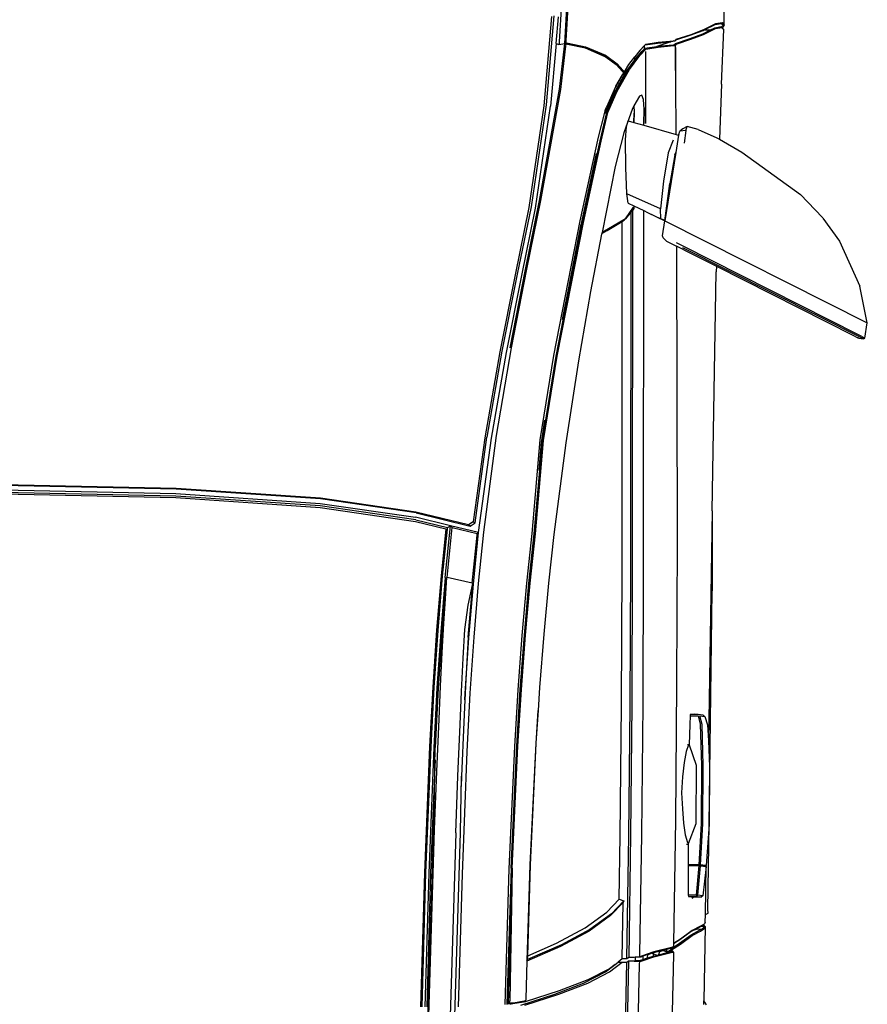
# Model space of a CAD drawing. Units: inches. Extents: x 0 to 4258, y 0 to 3769.
# Tile 11 of 30: x 3761 to 3796, y 3042 to 3082. Entities that reach past the tile are written whole.
import ezdxf

# ---------------------------------------------------------------- set-up
doc = ezdxf.new("R2010")
doc.units = ezdxf.units.IN
doc.header["$MEASUREMENT"] = 0
doc.layers.get('0').update_dxf_attribs({"color": 16})
doc.layers.add('C-PKNG-VEHI', color=8, linetype='Continuous', lineweight=18)
doc.layers.add('Edges', color=250, linetype='Continuous')

# ---------------------------------------------------------------- blocks, each defined once
blk = doc.blocks.new('Nissan Qashqai pl')
at = {"layer": 'Edges'}
for p, q in [((8.8918, 12.7444), (9.0186, 12.9956)), ((9.0386, 12.9907), (8.9254, 12.7664)), ((9.0186, 12.9956), (8.9731, 12.9865)), ((9.0374, 12.9925), (9.0186, 12.9956)), ((9.0356, 12.9888), (9.0333, 12.9845)), ((9.0356, 12.9888), (9.0374, 12.9925)), ((9.0386, 12.9907), (9.0374, 12.9925)), ((9.0376, 12.985), (9.0386, 12.9907)), ((8.9173, 12.961), (8.9731, 12.9865)), ((9.0333, 12.9845), (8.9232, 12.7662)), ((8.9483, 12.8082), (9.0343, 12.9785)), ((9.0343, 12.9785), (9.0347, 12.9794)), ((9.0347, 12.9794), (9.0362, 12.9822)), ((9.0362, 12.9822), (9.037, 12.9838)), ((9.0371, 12.9841), (9.037, 12.9838)), ((9.0371, 12.9841), (9.0376, 12.985)), ((9.0376, 12.985), (9.0371, 12.9847)), ((8.8885, 12.9405), (8.9173, 12.961)), ((8.8591, 12.9127), (8.8879, 12.94)), ((8.8885, 12.9405), (8.8879, 12.94)), ((8.8066, 12.84), (8.8591, 12.9127)), ((8.7908, 12.812), (8.8066, 12.84)), ((8.6489, 12.8179), (8.5719, 12.8193)), ((8.646, 12.8153), (8.6489, 12.8179)), ((8.6489, 12.8179), (8.6527, 12.8156)), ((8.6547, 12.8176), (8.6537, 12.8167)), ((8.7222, 12.8144), (8.6547, 12.8176)), ((8.646, 12.8153), (8.646, 12.8153)), ((8.6472, 12.8076), (8.646, 12.8153)), ((8.647, 12.8142), (8.6498, 12.8168)), ((8.6482, 12.8067), (8.647, 12.8142)), ((8.6546, 12.7926), (8.6472, 12.8076)), ((8.655, 12.7929), (8.6482, 12.8067)), ((8.6498, 12.8168), (8.6524, 12.8153)), ((8.651, 12.814), (8.652, 12.815)), ((8.6524, 12.8064), (8.651, 12.814)), ((8.652, 12.815), (8.6524, 12.8153)), ((8.6534, 12.8073), (8.652, 12.815)), ((8.6524, 12.8153), (8.6527, 12.8156)), ((8.655, 12.801), (8.6524, 12.8064)), ((8.6527, 12.8156), (8.6537, 12.8167)), ((8.6608, 12.7921), (8.6534, 12.8073)), ((8.6537, 12.8167), (8.6537, 12.8166)), ((8.7222, 12.8144), (8.7908, 12.812)), ((8.7785, 12.7855), (8.7891, 12.8089)), ((8.7891, 12.8089), (8.7908, 12.812)), ((8.928, 12.7679), (8.9483, 12.8082)), ((8.9483, 12.8082), (8.9552, 12.8081)), ((9.2517, 12.8031), (8.9552, 12.8081)), ((8.6606, 12.7768), (8.6546, 12.7926)), ((8.6598, 12.7913), (8.655, 12.801)), ((8.655, 12.7929), (8.655, 12.801)), ((8.6556, 12.7918), (8.655, 12.7929)), ((8.655, 12.7922), (8.655, 12.7929)), ((9.2517, 12.8031), (9.351, 12.803)), ((9.2517, 12.8031), (9.5372, 12.7983)), ((9.641, 12.7991), (9.351, 12.803)), ((9.5052, 12.7918), (9.5069, 12.7941)), ((9.5061, 12.7878), (9.5069, 12.7941)), ((9.5069, 12.7941), (9.5176, 12.7972)), ((9.5176, 12.7972), (9.5372, 12.7983)), ((9.5372, 12.7983), (9.5689, 12.7999)), ((9.5689, 12.7999), (9.641, 12.7991)), ((9.641, 12.7991), (9.6921, 12.7956)), ((9.7466, 12.7978), (9.641, 12.7991)), ((9.692, 12.7943), (9.6913, 12.7886)), ((9.6921, 12.7956), (9.692, 12.7943)), ((9.6922, 12.7943), (9.692, 12.7943)), ((9.6922, 12.7943), (9.6921, 12.7956)), ((9.7526, 12.7946), (9.6921, 12.7956)), ((9.6922, 12.7885), (9.693, 12.7955)), ((9.6922, 12.7885), (9.6922, 12.7943)), ((9.693, 12.7955), (9.7296, 12.7914)), ((9.7511, 12.7979), (9.7466, 12.7978)), ((9.7526, 12.7946), (9.7511, 12.7979)), ((9.7623, 12.7945), (9.7526, 12.7946)), ((9.7623, 12.7945), (9.7643, 12.7937)), ((9.7643, 12.7937), (9.7652, 12.7927)), ((9.7643, 12.7937), (9.7648, 12.7929)), ((9.7648, 12.7929), (9.7648, 12.7929)), ((9.7648, 12.7929), (9.7664, 12.7902)), ((9.7652, 12.7927), (9.7665, 12.7907)), ((9.7667, 12.7933), (9.7665, 12.7907)), ((9.7677, 12.7944), (9.7667, 12.7933)), ((9.7676, 12.7931), (9.7667, 12.7933)), ((9.7673, 12.7899), (9.7676, 12.7931)), ((9.769, 12.7926), (9.7676, 12.7931)), ((9.7677, 12.7944), (9.7677, 12.7944)), ((9.77, 12.7936), (9.7677, 12.7944)), ((9.7677, 12.7944), (9.8598, 12.7928)), ((9.7712, 12.7892), (9.769, 12.7926)), ((9.7734, 12.7884), (9.77, 12.7936)), ((9.8598, 12.7928), (9.8614, 12.7937)), ((9.8643, 12.7927), (9.8598, 12.7928)), ((9.8614, 12.7937), (9.8647, 12.7956)), ((8.6616, 12.7758), (8.6556, 12.7918)), ((8.6657, 12.7758), (8.6598, 12.7913)), ((8.6667, 12.7767), (8.6608, 12.7921)), ((8.7785, 12.7855), (8.7751, 12.7719)), ((9.5037, 12.7806), (9.5045, 12.7814)), ((9.5052, 12.7918), (9.5044, 12.7856)), ((9.5044, 12.7856), (9.5045, 12.7814)), ((9.5045, 12.7814), (9.5045, 12.7759)), ((9.5168, 12.7904), (9.5061, 12.7878)), ((9.5061, 12.7856), (9.5167, 12.7883)), ((9.5063, 12.7755), (9.5061, 12.7856)), ((9.5167, 12.7883), (9.5679, 12.7899)), ((9.5679, 12.792), (9.5168, 12.7904)), ((9.5678, 12.7837), (9.5426, 12.7747)), ((9.64, 12.7831), (9.5678, 12.7837)), ((9.6401, 12.7914), (9.5679, 12.792)), ((9.5679, 12.7899), (9.64, 12.7892)), ((9.64, 12.7892), (9.6912, 12.7865)), ((9.6645, 12.7737), (9.64, 12.7831)), ((9.6913, 12.7886), (9.6401, 12.7914)), ((9.6912, 12.7811), (9.6911, 12.7796)), ((9.6913, 12.7886), (9.6912, 12.7865)), ((9.6912, 12.7865), (9.6912, 12.7811)), ((9.692, 12.7811), (9.6912, 12.7811)), ((9.692, 12.7811), (9.6921, 12.7864)), ((9.692, 12.7796), (9.692, 12.7811)), ((9.6922, 12.7885), (9.6921, 12.7864)), ((9.6921, 12.7864), (9.7288, 12.7832)), ((9.7288, 12.7854), (9.6922, 12.7885)), ((9.7288, 12.7832), (9.7287, 12.7734)), ((9.7296, 12.7914), (9.7288, 12.7854)), ((9.7306, 12.7834), (9.7288, 12.7854)), ((9.7288, 12.7854), (9.7288, 12.7832)), ((9.7288, 12.7832), (9.7306, 12.7834)), ((9.7296, 12.7914), (9.7314, 12.7895)), ((9.7305, 12.7738), (9.7306, 12.7834)), ((9.7306, 12.7834), (9.7314, 12.7895)), ((9.7314, 12.7895), (9.7313, 12.7798)), ((9.7665, 12.7904), (9.7664, 12.7902)), ((9.7664, 12.7902), (9.7674, 12.7885)), ((9.7665, 12.7907), (9.7676, 12.7889)), ((9.7673, 12.7897), (9.7673, 12.7899)), ((9.7673, 12.7897), (9.7676, 12.7889)), ((9.7674, 12.7885), (9.7728, 12.7781)), ((9.7676, 12.7889), (9.7684, 12.7875)), ((9.7676, 12.7887), (9.7678, 12.7882)), ((9.7684, 12.7875), (9.7717, 12.781)), ((9.7707, 12.7848), (9.7709, 12.7893)), ((9.7717, 12.781), (9.7707, 12.7848)), ((9.7709, 12.7893), (9.7712, 12.7892)), ((9.7724, 12.7874), (9.7712, 12.7892)), ((9.7717, 12.781), (9.7738, 12.7771)), ((9.7778, 12.777), (9.7724, 12.7874)), ((9.7788, 12.778), (9.7734, 12.7884)), ((8.6667, 12.7584), (8.6606, 12.7768)), ((8.6675, 12.758), (8.6616, 12.7758)), ((8.6718, 12.7574), (8.6657, 12.7758)), ((8.6728, 12.7584), (8.6667, 12.7767)), ((8.7751, 12.7719), (8.7779, 12.7668)), ((8.7798, 12.7703), (8.7751, 12.7719)), ((8.7798, 12.7703), (8.7807, 12.763)), ((8.7798, 12.7703), (8.7954, 12.7683)), ((9.5045, 12.7759), (9.5063, 12.7755)), ((9.5063, 12.7755), (9.5168, 12.7751)), ((9.5168, 12.7751), (9.5423, 12.7746)), ((9.5423, 12.7746), (9.5422, 12.7736)), ((9.5422, 12.7736), (9.5422, 12.7725)), ((9.5422, 12.7736), (9.5424, 12.7735)), ((9.5426, 12.7747), (9.5423, 12.7746)), ((9.5426, 12.7747), (9.5424, 12.7735)), ((9.5424, 12.7735), (9.5503, 12.7706)), ((9.5503, 12.7706), (9.5641, 12.7681)), ((9.6395, 12.7676), (9.654, 12.7697)), ((9.654, 12.7697), (9.6633, 12.7726)), ((9.6633, 12.7726), (9.6645, 12.7737)), ((9.6655, 12.7733), (9.6645, 12.7737)), ((9.6655, 12.7733), (9.6911, 12.7732)), ((9.6655, 12.7713), (9.6655, 12.7733)), ((9.6911, 12.7796), (9.6911, 12.7732)), ((9.6911, 12.7732), (9.692, 12.7733)), ((9.692, 12.7733), (9.692, 12.7796)), ((9.692, 12.7733), (9.7287, 12.7734)), ((9.7287, 12.7734), (9.7305, 12.7738)), ((9.7305, 12.7738), (9.7313, 12.7798)), ((9.733, 12.7782), (9.7313, 12.7798)), ((9.7728, 12.7781), (9.7832, 12.7637)), ((9.7738, 12.7771), (9.7842, 12.7627)), ((9.7883, 12.7626), (9.7778, 12.777)), ((9.7894, 12.7636), (9.7788, 12.778)), ((8.6675, 12.758), (8.6667, 12.7584)), ((8.6679, 12.7578), (8.6675, 12.758)), ((8.6676, 12.7576), (8.6675, 12.7576)), ((8.6675, 12.7576), (8.6675, 12.7576)), ((8.6675, 12.7576), (8.6676, 12.7576)), ((8.6676, 12.7576), (8.6677, 12.7576)), ((8.6677, 12.7576), (8.6677, 12.7576)), ((8.6677, 12.7576), (8.6682, 12.7576)), ((8.6682, 12.7576), (8.6679, 12.7578)), ((8.6682, 12.7576), (8.6692, 12.7566)), ((8.6682, 12.7572), (8.6682, 12.7576)), ((8.6684, 12.7554), (8.6682, 12.7572)), ((8.6682, 12.7572), (8.6692, 12.7566)), ((8.6692, 12.7566), (8.6697, 12.7519)), ((8.6729, 12.7568), (8.6718, 12.7574)), ((8.674, 12.7578), (8.6728, 12.7584)), ((8.6733, 12.7566), (8.6729, 12.7568)), ((8.6735, 12.7544), (8.6733, 12.7566)), ((8.6742, 12.7576), (8.674, 12.7578)), ((8.6742, 12.7584), (8.6743, 12.7582)), ((8.6744, 12.755), (8.6742, 12.7576)), ((8.6744, 12.7576), (8.6742, 12.7576)), ((8.6744, 12.7578), (8.6744, 12.7576)), ((8.6773, 12.7577), (8.6744, 12.7576)), ((8.6791, 12.7578), (8.677, 12.7578)), ((8.6791, 12.7577), (8.6773, 12.7577)), ((8.7205, 12.7579), (8.6791, 12.7578)), ((8.6791, 12.7577), (8.6791, 12.7578)), ((8.6878, 12.7577), (8.6791, 12.7578)), ((8.6878, 12.7577), (8.6791, 12.7577)), ((8.6878, 12.7577), (8.6878, 12.7577)), ((8.6911, 12.7577), (8.6878, 12.7577)), ((8.7205, 12.7579), (8.6911, 12.7577)), ((8.7849, 12.7582), (8.7205, 12.7579)), ((8.7734, 12.7181), (8.7849, 12.7582)), ((8.7779, 12.7668), (8.7807, 12.763)), ((8.7849, 12.7615), (8.7807, 12.763)), ((8.7849, 12.7615), (8.7858, 12.7613)), ((8.7849, 12.7582), (8.7856, 12.7608)), ((8.7858, 12.7613), (8.7856, 12.7608)), ((8.7858, 12.7613), (8.807, 12.758)), ((8.8102, 12.7568), (8.807, 12.758)), ((8.807, 12.758), (8.8918, 12.7444)), ((8.8102, 12.7568), (8.8455, 12.7506)), ((8.9171, 12.7464), (8.9233, 12.7586)), ((8.9232, 12.7662), (8.9194, 12.7588)), ((8.925, 12.762), (8.9233, 12.7586)), ((8.9233, 12.7586), (9.2886, 12.7594)), ((8.928, 12.7679), (8.925, 12.762)), ((9.2886, 12.7594), (9.4673, 12.7589)), ((9.4673, 12.7589), (9.6358, 12.7575)), ((9.5641, 12.7681), (9.5818, 12.766)), ((9.5818, 12.766), (9.6016, 12.7651)), ((9.6016, 12.7651), (9.6215, 12.766)), ((9.6215, 12.766), (9.6395, 12.7676)), ((9.6358, 12.7575), (9.7887, 12.7552)), ((9.7832, 12.7637), (9.7887, 12.7552)), ((9.7842, 12.7627), (9.7891, 12.7552)), ((9.7933, 12.7549), (9.7883, 12.7626)), ((9.7965, 12.7526), (9.7894, 12.7636)), ((8.6684, 12.7554), (8.6685, 12.7549)), ((8.6684, 12.755), (8.6684, 12.7554)), ((8.6703, 12.7361), (8.6684, 12.755)), ((8.6697, 12.7519), (8.6698, 12.7516)), ((8.6714, 12.7353), (8.6697, 12.7519)), ((8.6698, 12.7516), (8.6755, 12.7343)), ((8.6754, 12.7353), (8.6735, 12.7544)), ((8.6764, 12.736), (8.6744, 12.755)), ((8.7917, 12.7547), (8.8075, 12.7486)), ((8.8075, 12.7486), (8.8429, 12.7426)), ((8.8918, 12.7444), (8.8455, 12.7506)), ((8.8815, 12.7228), (8.892, 12.7444)), ((8.892, 12.7444), (8.8908, 12.7421)), ((8.8911, 12.7428), (8.8919, 12.7444)), ((8.8911, 12.7428), (8.8919, 12.7444)), ((8.8919, 12.7444), (8.8911, 12.7428)), ((8.8919, 12.7444), (8.8918, 12.7444)), ((8.892, 12.7444), (8.8919, 12.7444)), ((8.8919, 12.7444), (8.8919, 12.7444)), ((8.8919, 12.7444), (8.8919, 12.7444)), ((8.9106, 12.7413), (8.892, 12.7444)), ((8.892, 12.7444), (8.892, 12.7444)), ((8.9171, 12.7464), (8.9131, 12.7421)), ((8.9171, 12.7464), (8.917, 12.7468)), ((9.7887, 12.7552), (9.7891, 12.7552)), ((9.7891, 12.7552), (9.79, 12.7552)), ((9.79, 12.7552), (9.7931, 12.7552)), ((9.7931, 12.7552), (9.7934, 12.7535)), ((9.7931, 12.7552), (9.7933, 12.7549)), ((9.7933, 12.7549), (9.7941, 12.7541)), ((9.7934, 12.7535), (9.7938, 12.7538)), ((9.7934, 12.7535), (9.7937, 12.7524)), ((9.7937, 12.7524), (9.7992, 12.7308)), ((9.7941, 12.7541), (9.7943, 12.7535)), ((9.7955, 12.7516), (9.7943, 12.7535)), ((9.7943, 12.7535), (9.7964, 12.7453)), ((9.7963, 12.7523), (9.7955, 12.7516)), ((9.7963, 12.7523), (9.7963, 12.7524)), ((9.7964, 12.7524), (9.7963, 12.7523)), ((9.7992, 12.7476), (9.7963, 12.7523)), ((9.7967, 12.7526), (9.7964, 12.7524)), ((9.7964, 12.7525), (9.7964, 12.7524)), ((9.7964, 12.7524), (9.7996, 12.7475)), ((9.7964, 12.7453), (9.7992, 12.7476)), ((9.7964, 12.7453), (9.7973, 12.7418)), ((9.7983, 12.7541), (9.7965, 12.7526)), ((9.7965, 12.7526), (9.7967, 12.7526)), ((9.7977, 12.7535), (9.7967, 12.7526)), ((9.7967, 12.7526), (9.7986, 12.7526)), ((9.7982, 12.754), (9.7977, 12.7535)), ((9.7977, 12.7444), (9.7985, 12.7451)), ((9.7985, 12.7451), (9.7977, 12.7431)), ((9.7977, 12.7431), (9.7977, 12.7444)), ((9.7983, 12.7541), (9.7982, 12.754)), ((9.7986, 12.7526), (9.7982, 12.754)), ((9.7986, 12.7544), (9.7983, 12.7541)), ((9.7989, 12.7461), (9.7985, 12.7451)), ((9.7993, 12.755), (9.7986, 12.7544)), ((9.7988, 12.7516), (9.7986, 12.7526)), ((9.7998, 12.7477), (9.7988, 12.7516)), ((9.7998, 12.7466), (9.7989, 12.7461)), ((9.7998, 12.7466), (9.7992, 12.7476)), ((9.7999, 12.7522), (9.7993, 12.755)), ((9.7993, 12.755), (9.8024, 12.7549)), ((9.7996, 12.7475), (9.7998, 12.7477)), ((9.8002, 12.7461), (9.7996, 12.7475)), ((9.8001, 12.7468), (9.7996, 12.7475)), ((9.8001, 12.7468), (9.7998, 12.7477)), ((9.8003, 12.7458), (9.7998, 12.7466)), ((9.8054, 12.7307), (9.7999, 12.7522)), ((9.8002, 12.7461), (9.8001, 12.7468)), ((9.8003, 12.7458), (9.8002, 12.7461)), ((9.8027, 12.7364), (9.8003, 12.7458)), ((9.8024, 12.7549), (9.9426, 12.7518)), ((8.6727, 12.7207), (8.6703, 12.7361)), ((8.6737, 12.7197), (8.6714, 12.7353)), ((8.6755, 12.7343), (8.6754, 12.7353)), ((8.6777, 12.7196), (8.6755, 12.7343)), ((8.6764, 12.7359), (8.6764, 12.736)), ((8.6788, 12.7205), (8.6764, 12.7359)), ((8.8429, 12.7426), (8.8771, 12.7388)), ((8.8771, 12.7388), (8.8585, 12.6969)), ((8.8895, 12.7393), (8.8771, 12.7388)), ((8.8815, 12.7228), (8.8895, 12.7393)), ((8.8908, 12.7421), (8.8895, 12.7393)), ((8.8906, 12.7418), (8.8895, 12.7393)), ((8.8906, 12.7418), (8.8911, 12.7428)), ((8.9131, 12.7421), (8.9106, 12.7413)), ((9.7977, 12.7431), (9.7973, 12.7418)), ((9.7973, 12.7418), (9.7977, 12.7409)), ((9.7973, 12.7418), (9.7977, 12.7399)), ((9.7977, 12.7399), (9.7977, 12.7409)), ((9.7977, 12.7409), (9.7987, 12.7388)), ((9.7977, 12.7399), (9.7978, 12.7397)), ((9.7987, 12.7388), (9.7978, 12.7397)), ((9.7978, 12.7397), (9.7987, 12.7362)), ((9.7987, 12.7388), (9.7992, 12.7377)), ((9.7987, 12.7362), (9.7992, 12.7377)), ((9.7987, 12.7362), (9.8002, 12.7301)), ((9.7992, 12.7377), (9.8027, 12.7364)), ((9.8014, 12.7303), (9.8031, 12.7349)), ((9.8031, 12.7349), (9.8027, 12.7364)), ((9.8043, 12.7303), (9.8031, 12.7349)), ((8.6737, 12.7197), (8.6727, 12.7207)), ((8.6746, 12.7189), (8.6737, 12.7197)), ((8.6785, 12.7189), (8.6777, 12.7196)), ((8.687, 12.7132), (8.6788, 12.7205)), ((8.6818, 12.7204), (8.7012, 12.7203)), ((8.7012, 12.7203), (8.7012, 12.7203)), ((8.7012, 12.7203), (8.7026, 12.7203)), ((8.7026, 12.7203), (8.7026, 12.7203)), ((8.7026, 12.7203), (8.7072, 12.7203)), ((8.7072, 12.7203), (8.7072, 12.7203)), ((8.7072, 12.7203), (8.7273, 12.7202)), ((8.7273, 12.7202), (8.7273, 12.7201)), ((8.7273, 12.7202), (8.7354, 12.7202)), ((8.7354, 12.7201), (8.7354, 12.7202)), ((8.7354, 12.7202), (8.742, 12.7202)), ((8.742, 12.7201), (8.742, 12.7202)), ((8.742, 12.7202), (8.742, 12.7201)), ((8.742, 12.7202), (8.742, 12.7202)), ((8.742, 12.7202), (8.7426, 12.7202)), ((8.7426, 12.7201), (8.7426, 12.7202)), ((8.7426, 12.7202), (8.7433, 12.7202)), ((8.7433, 12.7201), (8.7433, 12.7202)), ((8.7433, 12.7202), (8.7711, 12.7201)), ((8.7711, 12.7201), (8.7516, 12.72)), ((8.8793, 12.7181), (8.8815, 12.7228)), ((9.7992, 12.7308), (9.8044, 12.7151)), ((9.8002, 12.7301), (9.8008, 12.7285)), ((9.8008, 12.7285), (9.8014, 12.7303)), ((9.8008, 12.7285), (9.8014, 12.7265)), ((9.8043, 12.7303), (9.8014, 12.7303)), ((9.8014, 12.7265), (9.803, 12.723)), ((9.8014, 12.7265), (9.8026, 12.723)), ((9.803, 12.723), (9.8026, 12.723)), ((9.8026, 12.723), (9.8046, 12.7171)), ((9.8067, 12.7229), (9.803, 12.723)), ((9.8044, 12.73), (9.8043, 12.7303)), ((9.8067, 12.7229), (9.8044, 12.73)), ((9.8106, 12.715), (9.8054, 12.7307)), ((9.8086, 12.7171), (9.8067, 12.7229)), ((8.6785, 12.7189), (8.6746, 12.7189)), ((8.6805, 12.7132), (8.6746, 12.7189)), ((8.6815, 12.7162), (8.6785, 12.7189)), ((8.6805, 12.7132), (8.6884, 12.7071)), ((8.6815, 12.7162), (8.6818, 12.7154)), ((8.6817, 12.716), (8.6815, 12.7162)), ((8.6817, 12.716), (8.6818, 12.7154)), ((8.6859, 12.7122), (8.6817, 12.716)), ((8.6818, 12.7154), (8.6902, 12.7081)), ((8.6927, 12.7071), (8.6859, 12.7122)), ((8.7042, 12.7002), (8.687, 12.7132)), ((8.6917, 12.7071), (8.6884, 12.7071)), ((8.698, 12.6996), (8.6884, 12.7071)), ((8.6902, 12.7081), (8.6917, 12.7071)), ((8.6917, 12.7071), (8.7075, 12.6955)), ((8.6927, 12.7071), (8.6923, 12.7071)), ((8.7032, 12.6992), (8.6927, 12.7071)), ((8.7415, 12.7177), (8.7361, 12.7158)), ((8.7361, 12.7158), (8.7373, 12.7128)), ((8.7373, 12.7128), (8.7492, 12.7059)), ((8.7534, 12.7185), (8.7415, 12.7177)), ((8.7718, 12.7181), (8.7534, 12.7185)), ((8.7698, 12.7058), (8.7734, 12.7181)), ((8.7734, 12.7181), (8.7718, 12.7181)), ((8.8734, 12.7057), (8.8793, 12.7181)), ((9.3194, 12.7179), (8.8793, 12.7181)), ((9.4919, 12.7173), (9.3194, 12.7179)), ((9.6538, 12.7157), (9.4919, 12.7173)), ((9.802, 12.7133), (9.6538, 12.7157)), ((9.8051, 12.7132), (9.802, 12.7133)), ((9.8044, 12.7151), (9.8051, 12.7132)), ((9.8046, 12.7171), (9.8086, 12.7171)), ((9.8046, 12.7171), (9.8055, 12.7143)), ((9.8061, 12.6994), (9.8051, 12.7132)), ((9.8055, 12.7143), (9.8058, 12.7073)), ((9.8058, 12.7073), (9.8098, 12.7073)), ((9.8058, 12.7073), (9.8061, 12.6994)), ((9.8096, 12.7142), (9.8086, 12.7171)), ((9.8098, 12.7073), (9.8096, 12.7142)), ((9.8101, 12.6993), (9.8098, 12.7073)), ((9.8101, 12.6993), (9.8112, 12.7131)), ((9.8112, 12.7131), (9.8106, 12.715)), ((9.8143, 12.713), (9.8112, 12.7131)), ((9.9414, 12.71), (9.8143, 12.713)), ((8.7071, 12.6942), (8.698, 12.6996)), ((8.7302, 12.684), (8.7032, 12.6992)), ((8.7312, 12.6851), (8.7042, 12.7002)), ((8.7075, 12.6955), (8.7346, 12.6806)), ((8.7492, 12.7059), (8.7572, 12.7062)), ((8.7492, 12.7059), (8.7524, 12.704)), ((8.7524, 12.704), (8.7828, 12.6934)), ((8.7572, 12.7062), (8.7698, 12.7058)), ((8.7698, 12.7057), (8.7583, 12.706)), ((8.7678, 12.6988), (8.7698, 12.7057)), ((8.7748, 12.6967), (8.7678, 12.6988)), ((8.7698, 12.7057), (8.7698, 12.7058)), ((8.7916, 12.6954), (8.7748, 12.6967)), ((8.8259, 12.6959), (8.7916, 12.6954)), ((8.8585, 12.6969), (8.8259, 12.6959)), ((8.87, 12.6987), (8.8585, 12.6969)), ((8.87, 12.6987), (8.8734, 12.7057)), ((8.8734, 12.7057), (8.8768, 12.7057)), ((8.8751, 12.7054), (8.8768, 12.7057)), ((8.8893, 12.6956), (8.8751, 12.7054)), ((8.8768, 12.7057), (8.879, 12.704)), ((8.879, 12.704), (9.3198, 12.7039)), ((8.879, 12.704), (8.881, 12.7023)), ((9.3225, 12.7021), (8.881, 12.7023)), ((8.881, 12.7023), (8.8893, 12.6956)), ((8.8893, 12.6956), (8.9021, 12.6745)), ((8.8913, 12.6936), (8.8893, 12.6956)), ((9.3198, 12.7039), (9.4922, 12.7033)), ((9.4936, 12.7013), (9.3225, 12.7021)), ((9.4922, 12.7033), (9.654, 12.7018)), ((9.6552, 12.6997), (9.4936, 12.7013)), ((9.654, 12.7018), (9.8061, 12.6994)), ((9.8078, 12.6971), (9.6552, 12.6997)), ((9.8061, 12.6994), (9.8078, 12.6971)), ((9.8078, 12.6971), (9.8078, 12.6913)), ((9.8119, 12.697), (9.8101, 12.6993)), ((9.8101, 12.6993), (9.9411, 12.6966)), ((9.9393, 12.6944), (9.8119, 12.697)), ((9.8119, 12.6912), (9.8119, 12.697)), ((8.6864, 12.6706), (8.697, 12.685)), ((8.6875, 12.6698), (8.6979, 12.6839)), ((8.6987, 12.6845), (8.6924, 12.676)), ((8.697, 12.685), (8.7055, 12.6927)), ((8.6979, 12.6839), (8.7062, 12.6915)), ((8.7062, 12.6915), (8.6987, 12.6845)), ((8.7055, 12.6927), (8.7071, 12.6942)), ((8.7062, 12.6915), (8.7067, 12.6919)), ((8.7067, 12.6919), (8.7083, 12.6934)), ((8.7071, 12.6942), (8.7083, 12.6934)), ((8.7083, 12.6934), (8.7083, 12.6934)), ((8.7083, 12.6934), (8.7083, 12.6934)), ((8.7102, 12.6923), (8.7083, 12.6934)), ((8.7083, 12.6934), (8.7083, 12.6934)), ((8.7108, 12.6919), (8.7102, 12.6923)), ((8.7102, 12.6923), (8.7102, 12.6923)), ((8.7257, 12.6833), (8.7108, 12.6919)), ((8.7248, 12.6836), (8.7108, 12.6919)), ((8.7257, 12.6833), (8.7248, 12.6836)), ((8.7257, 12.6832), (8.7257, 12.6833)), ((8.7257, 12.6832), (8.7508, 12.672)), ((8.7529, 12.6741), (8.7302, 12.684)), ((8.7574, 12.6737), (8.7312, 12.6851)), ((8.7828, 12.6934), (8.8245, 12.6828)), ((8.8245, 12.6828), (8.9063, 12.6663)), ((8.8927, 12.6913), (8.8913, 12.6936)), ((9.3224, 12.6911), (8.8927, 12.6913)), ((8.9041, 12.6725), (8.8927, 12.6913)), ((9.3225, 12.6911), (9.3224, 12.6911)), ((9.4936, 12.6904), (9.3225, 12.6911)), ((9.6552, 12.6888), (9.4936, 12.6904)), ((9.7337, 12.6875), (9.6552, 12.6888)), ((9.7337, 12.6875), (9.7357, 12.6935)), ((9.7499, 12.6721), (9.7337, 12.6875)), ((9.7357, 12.6935), (9.7378, 12.6924)), ((9.7357, 12.6935), (9.7519, 12.678)), ((9.7378, 12.6924), (9.754, 12.677)), ((9.8078, 12.6913), (9.7378, 12.6924)), ((9.8078, 12.6913), (9.8119, 12.6862)), ((9.8241, 12.6756), (9.8119, 12.6912)), ((9.8119, 12.6862), (9.8119, 12.6912)), ((9.8147, 12.6826), (9.8119, 12.6862)), ((8.6759, 12.6459), (8.6864, 12.6706)), ((8.6883, 12.6704), (8.6777, 12.6457)), ((8.6924, 12.676), (8.6883, 12.6704)), ((8.6924, 12.676), (8.6924, 12.6762)), ((8.7346, 12.6806), (8.7491, 12.6738)), ((8.7346, 12.6806), (8.7577, 12.6709)), ((8.7508, 12.672), (8.7491, 12.6738)), ((8.7491, 12.6738), (8.7576, 12.6699)), ((8.7532, 12.6708), (8.7508, 12.672)), ((8.7529, 12.6741), (8.7577, 12.6709)), ((8.757, 12.6724), (8.7529, 12.6741)), ((8.7575, 12.6698), (8.7532, 12.6708)), ((8.7587, 12.672), (8.757, 12.6724)), ((8.7931, 12.6653), (8.7574, 12.6737)), ((8.7582, 12.6707), (8.7576, 12.6699)), ((8.7577, 12.6709), (8.7582, 12.6707)), ((8.759, 12.6717), (8.7582, 12.6707)), ((8.7587, 12.672), (8.759, 12.6717)), ((8.7591, 12.6719), (8.7587, 12.672)), ((8.7591, 12.6719), (8.759, 12.6717)), ((8.7925, 12.664), (8.7591, 12.6719)), ((8.9021, 12.6745), (8.9063, 12.6663)), ((8.9075, 12.6661), (8.9041, 12.6725)), ((9.7692, 12.6453), (9.7499, 12.6721)), ((9.7519, 12.678), (9.7713, 12.6512)), ((9.754, 12.677), (9.7733, 12.6502)), ((9.8147, 12.6826), (9.8147, 12.6826)), ((9.8147, 12.6826), (9.8201, 12.6756)), ((9.8241, 12.6706), (9.8147, 12.6826)), ((9.8201, 12.6756), (9.8338, 12.6486)), ((9.8378, 12.6485), (9.8241, 12.6756)), ((9.8378, 12.6435), (9.8241, 12.6706)), ((8.6772, 12.6454), (8.6875, 12.6698)), ((8.7576, 12.6699), (8.7575, 12.6698)), ((8.7881, 12.6621), (8.7575, 12.6698)), ((8.8918, 12.6392), (8.7881, 12.6621)), ((8.8941, 12.6418), (8.7925, 12.664)), ((8.8942, 12.6432), (8.7931, 12.6653)), ((8.8083, 12.6591), (8.8954, 12.6403)), ((8.9063, 12.6663), (8.9075, 12.6661)), ((8.9075, 12.6661), (8.9087, 12.6658)), ((8.9087, 12.6658), (8.9797, 12.6518)), ((8.9797, 12.6518), (9.0656, 12.6372)), ((9.7713, 12.6512), (9.7905, 12.6158)), ((9.7733, 12.6502), (9.7925, 12.6148)), ((9.8338, 12.6486), (9.8475, 12.613)), ((9.8516, 12.6129), (9.8378, 12.6485)), ((8.6716, 12.6242), (8.6759, 12.6459)), ((8.6772, 12.6454), (8.6721, 12.6201)), ((8.6777, 12.6457), (8.6727, 12.6213)), ((8.9679, 12.6241), (8.8918, 12.6392)), ((9.0601, 12.6092), (8.8941, 12.6418)), ((8.9696, 12.6285), (8.8942, 12.6432)), ((8.8961, 12.6401), (8.9704, 12.6257)), ((9.0656, 12.6372), (9.1676, 12.6212)), ((9.7885, 12.6099), (9.7692, 12.6453)), ((9.8516, 12.6079), (9.8378, 12.6435)), ((8.6197, 12.6241), (8.6683, 12.6215)), ((8.6721, 12.6201), (8.6204, 12.6229)), ((8.6683, 12.6215), (8.671, 12.6214)), ((8.671, 12.6214), (8.6716, 12.6242)), ((9.0591, 12.6065), (8.9679, 12.6241)), ((9.06, 12.6106), (8.9696, 12.6285)), ((8.9704, 12.6257), (8.9708, 12.6256)), ((8.9708, 12.6256), (9.0143, 12.6169)), ((8.622, 12.6161), (8.6699, 12.6132)), ((8.6721, 12.6093), (8.6387, 12.6123)), ((8.6699, 12.6132), (8.6721, 12.613)), ((8.671, 12.6214), (8.6721, 12.6201)), ((8.6727, 12.6213), (8.6721, 12.6201)), ((8.6733, 12.6129), (8.6721, 12.6201)), ((8.7287, 12.6134), (8.6721, 12.6201)), ((8.6721, 12.6127), (8.6721, 12.613)), ((8.6721, 12.613), (8.6733, 12.6129)), ((8.6721, 12.6093), (8.6733, 12.6129)), ((8.6721, 12.6093), (8.7496, 12.6025)), ((8.6727, 12.6213), (8.6753, 12.621)), ((8.6753, 12.621), (8.7292, 12.6146)), ((8.8666, 12.5888), (8.7287, 12.6134)), ((8.7292, 12.6146), (8.8666, 12.5901)), ((9.1644, 12.5938), (9.06, 12.6106)), ((9.1676, 12.6212), (9.2814, 12.6065)), ((9.8039, 12.5741), (9.7885, 12.6099)), ((9.7905, 12.6158), (9.8087, 12.574)), ((9.7925, 12.6148), (9.8107, 12.573)), ((9.8475, 12.613), (9.8611, 12.5708)), ((9.8652, 12.5704), (9.8516, 12.6129)), ((8.6375, 12.6066), (8.7481, 12.5968)), ((8.6386, 12.6037), (8.7491, 12.594)), ((8.8761, 12.5839), (8.7496, 12.6025)), ((9.1639, 12.5895), (9.0591, 12.6065)), ((9.1645, 12.5924), (9.0601, 12.6092)), ((9.2814, 12.6065), (9.3416, 12.5999)), ((9.3416, 12.5999), (9.4048, 12.5941)), ((9.8652, 12.5654), (9.8516, 12.6079)), ((8.7481, 12.5968), (8.8745, 12.5782)), ((8.7491, 12.594), (8.8754, 12.5755)), ((8.8666, 12.5901), (8.9521, 12.5726)), ((8.9522, 12.5713), (8.8666, 12.5888)), ((9.1393, 12.5951), (9.1647, 12.591)), ((9.2801, 12.5794), (9.1639, 12.5895)), ((9.2803, 12.5836), (9.1644, 12.5938)), ((9.2804, 12.5821), (9.1645, 12.5924)), ((9.1647, 12.591), (9.1668, 12.5908)), ((9.1668, 12.5908), (9.2019, 12.5877)), ((9.4048, 12.5941), (9.471, 12.5888)), ((9.471, 12.5888), (9.4997, 12.5869)), ((9.5404, 12.5844), (9.4997, 12.5869)), ((9.4997, 12.5869), (9.5403, 12.5842)), ((8.8745, 12.5782), (8.9583, 12.5609)), ((8.8754, 12.5755), (8.9591, 12.5583)), ((8.9598, 12.5666), (8.8761, 12.5839)), ((9.3418, 12.5729), (9.2801, 12.5794)), ((9.3418, 12.5771), (9.2803, 12.5836)), ((9.3419, 12.5756), (9.2804, 12.5821)), ((9.4062, 12.5713), (9.3418, 12.5771)), ((9.4064, 12.5671), (9.3418, 12.5729)), ((9.4063, 12.5699), (9.3419, 12.5756)), ((9.5403, 12.5842), (9.6913, 12.5767)), ((9.6912, 12.5774), (9.5404, 12.5844)), ((9.8039, 12.5741), (9.6912, 12.5774)), ((9.6913, 12.5767), (9.8099, 12.573)), ((9.8087, 12.574), (9.8039, 12.5741)), ((9.8099, 12.573), (9.8087, 12.574)), ((9.8099, 12.573), (9.8107, 12.573)), ((9.8107, 12.573), (9.8573, 12.5716)), ((8.9521, 12.5726), (9.0495, 12.5536)), ((9.0497, 12.5523), (8.9522, 12.5713)), ((8.9583, 12.5609), (9.0538, 12.5419)), ((9.0552, 12.5477), (8.9598, 12.5666)), ((9.4735, 12.5663), (9.4062, 12.5713)), ((9.4736, 12.5648), (9.4063, 12.5699)), ((9.4739, 12.5621), (9.4064, 12.5671)), ((9.5437, 12.5619), (9.4735, 12.5663)), ((9.5438, 12.5605), (9.4736, 12.5648)), ((9.5443, 12.5579), (9.4739, 12.5621)), ((9.6953, 12.5549), (9.5437, 12.5619)), ((9.6954, 12.5535), (9.5438, 12.5605)), ((9.8573, 12.5716), (9.8603, 12.5715)), ((9.8603, 12.5715), (9.8605, 12.5696)), ((9.8611, 12.5708), (9.8603, 12.5715)), ((9.8605, 12.5696), (9.8626, 12.5564)), ((9.8612, 12.5707), (9.8611, 12.5708)), ((9.8612, 12.5707), (9.8615, 12.5688)), ((9.8615, 12.5688), (9.8635, 12.5556)), ((8.9591, 12.5583), (9.0546, 12.5394)), ((9.0495, 12.5536), (9.1584, 12.5351)), ((9.696, 12.551), (9.5443, 12.5579)), ((9.6953, 12.5549), (9.8598, 12.5517)), ((9.6953, 12.5549), (9.863, 12.5497)), ((9.6954, 12.5535), (9.8641, 12.5483)), ((9.8644, 12.5459), (9.696, 12.551)), ((9.8629, 12.5516), (9.8598, 12.5517)), ((9.8626, 12.5564), (9.8627, 12.5532)), ((9.8637, 12.5532), (9.8627, 12.5532)), ((9.8627, 12.5532), (9.8629, 12.5516)), ((9.8629, 12.5516), (9.863, 12.5497)), ((9.8641, 12.5483), (9.863, 12.5497)), ((9.8635, 12.5556), (9.8637, 12.5532)), ((9.8643, 12.5532), (9.8637, 12.5532)), ((9.8637, 12.5532), (9.8638, 12.5508)), ((9.8638, 12.5508), (9.8641, 12.5483)), ((9.0538, 12.5419), (9.1605, 12.5233)), ((9.0546, 12.5394), (9.1612, 12.5208)), ((9.1617, 12.5292), (9.0552, 12.5477)), ((9.1584, 12.5351), (9.2783, 12.5191)), ((9.2789, 12.5131), (9.1617, 12.5292)), ((9.2669, 12.5088), (9.1605, 12.5233)), ((9.1612, 12.5208), (9.2656, 12.5065)), ((9.2789, 12.5131), (9.2704, 12.4783)), ((9.2783, 12.5191), (9.3422, 12.5126)), ((9.2799, 12.5114), (9.2789, 12.5131)), ((9.3427, 12.5066), (9.2789, 12.5131)), ((9.2803, 12.5116), (9.2822, 12.5118)), ((9.3422, 12.5126), (9.4088, 12.507)), ((9.2694, 12.5006), (9.2535, 12.4354)), ((9.2543, 12.4356), (9.2707, 12.5028)), ((9.2656, 12.5065), (9.2669, 12.5088)), ((9.2656, 12.5065), (9.2694, 12.5006)), ((9.2707, 12.5028), (9.2669, 12.5088)), ((9.2707, 12.5028), (9.2694, 12.5006)), ((9.2724, 12.4804), (9.2799, 12.5114)), ((9.2819, 12.5112), (9.2799, 12.5114)), ((9.3418, 12.5051), (9.2819, 12.5112)), ((9.3418, 12.5051), (9.3346, 12.4741)), ((9.342, 12.5059), (9.3418, 12.5051)), ((9.3687, 12.5), (9.342, 12.5059)), ((9.4087, 12.5003), (9.342, 12.5059)), ((9.4093, 12.5011), (9.3427, 12.5066)), ((9.3992, 12.496), (9.3687, 12.5)), ((9.4087, 12.5003), (9.4688, 12.4968)), ((9.4088, 12.507), (9.4782, 12.5024)), ((9.4785, 12.4965), (9.4093, 12.5011)), ((9.4782, 12.5024), (9.5503, 12.4987)), ((9.4347, 12.494), (9.3992, 12.496)), ((9.4761, 12.4919), (9.4347, 12.494)), ((9.4688, 12.4968), (9.4789, 12.4964)), ((9.5168, 12.4903), (9.4761, 12.4919)), ((9.4789, 12.4964), (9.4785, 12.4965)), ((9.4862, 12.4961), (9.4785, 12.4965)), ((9.4789, 12.4964), (9.4862, 12.4961)), ((9.4862, 12.4961), (9.514, 12.4949)), ((9.514, 12.4949), (9.5811, 12.492)), ((9.5812, 12.4874), (9.5168, 12.4903)), ((9.5503, 12.4987), (9.7029, 12.4926)), ((9.651, 12.4906), (9.5811, 12.492)), ((9.5811, 12.492), (9.594, 12.4914)), ((9.6514, 12.4849), (9.5812, 12.4874)), ((9.9583, 12.4812), (9.651, 12.4906)), ((9.7029, 12.4926), (9.8673, 12.4878)), ((9.2704, 12.4783), (9.2598, 12.4348)), ((9.2724, 12.4804), (9.2704, 12.4783)), ((9.2726, 12.4746), (9.2704, 12.4783)), ((9.3346, 12.4718), (9.2704, 12.4783)), ((9.3346, 12.4741), (9.2724, 12.4804)), ((9.6514, 12.4849), (9.9312, 12.4761)), ((9.2629, 12.435), (9.2726, 12.4746)), ((9.2649, 12.4348), (9.2741, 12.4725)), ((9.2746, 12.4744), (9.2726, 12.4746)), ((9.2741, 12.4725), (9.3326, 12.4666)), ((9.333, 12.4685), (9.2746, 12.4744)), ((9.3326, 12.4666), (9.4, 12.4609)), ((9.4004, 12.4629), (9.333, 12.4685)), ((9.3346, 12.4741), (9.3344, 12.4733)), ((9.3344, 12.4733), (9.4017, 12.4677)), ((9.3344, 12.4733), (9.3611, 12.4715)), ((9.3346, 12.4718), (9.4018, 12.4661)), ((9.3611, 12.4715), (9.3918, 12.4695)), ((9.3918, 12.4695), (9.4276, 12.4674)), ((9.4709, 12.4581), (9.4004, 12.4629)), ((9.4017, 12.4677), (9.472, 12.463)), ((9.4018, 12.4661), (9.472, 12.4614)), ((9.4276, 12.4674), (9.4694, 12.4654)), ((9.4694, 12.4654), (9.5105, 12.4637)), ((9.472, 12.463), (9.5454, 12.4591)), ((9.5105, 12.4637), (9.5755, 12.4608)), ((9.4, 12.4609), (9.4706, 12.4561)), ((9.4706, 12.4561), (9.5443, 12.4522)), ((9.5446, 12.4542), (9.4709, 12.4581)), ((9.472, 12.4614), (9.5454, 12.4576)), ((9.5443, 12.4522), (9.701, 12.4459)), ((9.7011, 12.4478), (9.5446, 12.4542)), ((9.5454, 12.4591), (9.5454, 12.4593)), ((9.5695, 12.4589), (9.5454, 12.4591)), ((9.5454, 12.4576), (9.7014, 12.4513)), ((9.5609, 12.4593), (9.5695, 12.4589)), ((9.5786, 12.4588), (9.5695, 12.4589)), ((9.5695, 12.4589), (9.7014, 12.4536)), ((9.5755, 12.4608), (9.6472, 12.4581)), ((9.6206, 12.4581), (9.5786, 12.4588)), ((9.6714, 12.4567), (9.6206, 12.4581)), ((9.6414, 12.458), (9.6407, 12.458)), ((9.6472, 12.4581), (9.9278, 12.4492)), ((9.6549, 12.4576), (9.6558, 12.4574)), ((9.6825, 12.4564), (9.6714, 12.4567)), ((9.6825, 12.4564), (9.6829, 12.4563)), ((9.6943, 12.456), (9.6825, 12.4564)), ((9.6943, 12.4558), (9.6943, 12.456)), ((9.6951, 12.456), (9.6943, 12.456)), ((9.6951, 12.4558), (9.6951, 12.456)), ((9.8565, 12.451), (9.6951, 12.456)), ((9.7014, 12.4536), (9.8673, 12.4488)), ((9.7014, 12.4513), (9.8673, 12.4464)), ((9.9794, 12.4475), (9.8565, 12.451)), ((9.701, 12.4459), (9.8673, 12.441)), ((9.8673, 12.443), (9.7011, 12.4478)), ((9.2535, 12.4354), (9.2362, 12.3167)), ((9.2543, 12.4356), (9.2371, 12.3169)), ((9.2426, 12.3164), (9.2598, 12.4348)), ((9.2629, 12.435), (9.2457, 12.3164)), ((9.2476, 12.3163), (9.2649, 12.4348)), ((9.2362, 12.3167), (9.2241, 12.1376)), ((9.2371, 12.3169), (9.2249, 12.1376)), ((9.2305, 12.1375), (9.2426, 12.3164)), ((9.2457, 12.3164), (9.2335, 12.1374)), ((9.2355, 12.1374), (9.2476, 12.3163)), ((9.2241, 12.1376), (9.2195, 11.9221)), ((9.2249, 12.1376), (9.2203, 11.9221)), ((9.2259, 11.9221), (9.2305, 12.1375)), ((9.2335, 12.1374), (9.2289, 11.9221)), ((9.2308, 11.9221), (9.2355, 12.1374))]:
    blk.add_line(p, q, dxfattribs=at)
blk = doc.blocks.new('car')
blk.add_blockref('Nissan Qashqai pl', (-9.7433, -11.9151))

msp = doc.modelspace()

# ---------------------------------------------------------------- block references
at = {"layer": 'C-PKNG-VEHI', "xscale": 32.66500240257601, "yscale": 32.66500240257601, "zscale": 32.66500240257601, "rotation": 270}
msp.add_blockref('car', (3760.419, 3045.57), dxfattribs=at)

doc.saveas('drawing.dxf')
